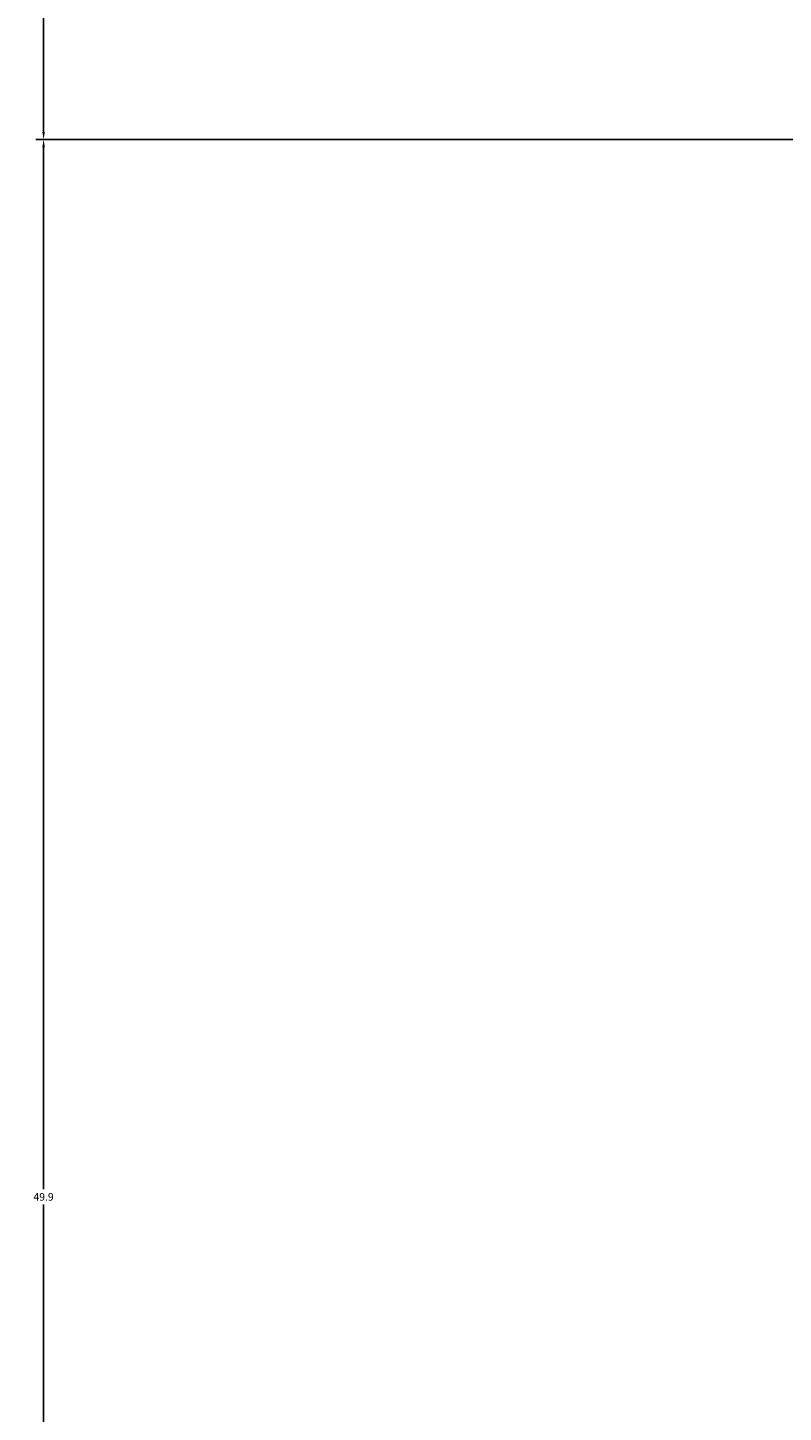
# Model space of a CAD drawing. Units: inches. Extents: x 738 to 1068, y 378 to 757.
# Tile 4 of 41: x 738 to 756, y 416 to 449. Entities that reach past the tile are written whole.
import ezdxf

# ---------------------------------------------------------------- set-up
doc = ezdxf.new("R2010")
doc.units = ezdxf.units.IN
doc.header["$MEASUREMENT"] = 0
doc.layers.add('A-ANNO-DIMS', color=2, linetype='Continuous', lineweight=18)
doc.styles.get("Standard").update_dxf_attribs({"font": 'arial.ttf'})
doc.dimstyles.get("Standard").update_dxf_attribs({"dimtxt": 0.18, "dimasz": 0.18, "dimexe": 0.18, "dimexo": 0.0625, "dimgap": 0.09, "dimtad": 0, "dimtih": 1, "dimtoh": 1, "dimdec": 4, "dimzin": 0, "dimdsep": 46, "dimtxsty": 'Standard', "dimcen": 0.09, "dimadec": 0, "dimazin": 0, "dimtfac": 1, "dimtdec": 4, "dimtofl": 0, "dimtmove": 0, "dimatfit": 3, "dimfxl": 1, "dimtolj": 1, "dimtzin": 0, "dimarcsym": 0})

# ---------------------------------------------------------------- blocks, each defined once
blk = doc.blocks.new('*D19')
at = {"layer": 'A-ANNO-DIMS', "color": 0, "lineweight": -2, "transparency": 16777216}
for p, q in [((781.422, 446.265), (738.194, 446.265)), ((738.374, 446.085), (738.374, 421.499)), ((738.374, 396.549), (738.374, 421.135)), ((781.385, 396.369), (738.194, 396.369))]:
    blk.add_line(p, q, dxfattribs=at)
at = {"layer": 'A-ANNO-DIMS', "color": 0, "transparency": 16777216}
for points in [[(738.344, 446.085), (738.404, 446.085), (738.374, 446.265)], [(738.344, 396.549), (738.404, 396.549), (738.374, 396.369)]]:
    blk.add_solid(points, dxfattribs=at)
at = {"layer": 'Defpoints', "color": 0, "transparency": 16777216}
for p in [(738.374, 446.265), (781.485, 446.265), (781.447, 396.369)]:
    blk.add_point(p, dxfattribs=at)
at = {"layer": 'A-ANNO-DIMS', "color": 0, "transparency": 16777216, "insert": (738.374, 421.317), "char_height": 0.18, "attachment_point": 5}
blk.add_mtext('\\A1;49.9', dxfattribs=at)
blk = doc.blocks.new('*D20')
at = {"layer": 'A-ANNO-DIMS', "color": 0, "lineweight": -2, "transparency": 16777216}
for p, q in [((781.427, 461.392), (738.194, 461.392)), ((738.374, 461.212), (738.374, 454.01)), ((738.374, 446.445), (738.374, 453.647)), ((781.422, 446.265), (738.194, 446.265))]:
    blk.add_line(p, q, dxfattribs=at)
at = {"layer": 'A-ANNO-DIMS', "color": 0, "transparency": 16777216}
for points in [[(738.344, 461.212), (738.404, 461.212), (738.374, 461.392)], [(738.344, 446.445), (738.404, 446.445), (738.374, 446.265)]]:
    blk.add_solid(points, dxfattribs=at)
at = {"layer": 'Defpoints', "color": 0, "transparency": 16777216}
for p in [(738.374, 461.392), (781.49, 461.392), (781.485, 446.265)]:
    blk.add_point(p, dxfattribs=at)
at = {"layer": 'A-ANNO-DIMS', "color": 0, "transparency": 16777216, "insert": (738.374, 453.829), "char_height": 0.18, "attachment_point": 5}
blk.add_mtext('\\A1;15.127', dxfattribs=at)

msp = doc.modelspace()

# ---------------------------------------------------------------- dimensions: what is measured, and where the dimension line sits
at = {"layer": 'A-ANNO-DIMS'}
for base, p1, p2, override, picture, middle in [((738.3736, 461.3919), (781.4846, 446.2651), (781.4897, 461.3919), {"dimdec": 3, "dimlfac": 1, "dimrnd": 0, "dimzin": 0, "dimdsep": 46, "dimlunit": 2}, '*D20', (738.3736, 453.8285)), ((738.3736, 446.2651), (781.4474, 396.3691), (781.4846, 446.2651), {"dimdec": 1, "dimlfac": 1, "dimrnd": 0, "dimzin": 0, "dimdsep": 46, "dimlunit": 2}, '*D19', (738.3736, 421.3171))]:
    dim = msp.add_linear_dim(base=base, p1=p1, p2=p2, angle=90, dimstyle='Standard', override=override, dxfattribs=at)
    dim.commit()
    dim.dimension.update_dxf_attribs({"geometry": picture, "text_midpoint": middle})

doc.saveas('drawing.dxf')
